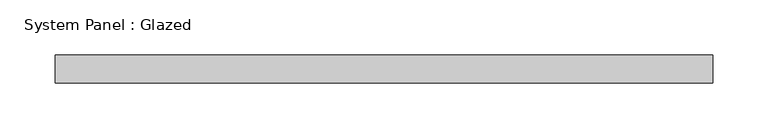
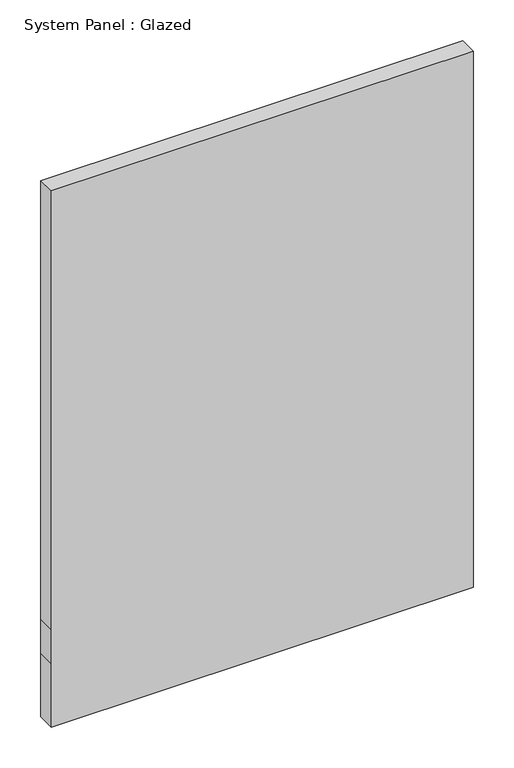
"""IFC4 building model written with IfcOpenShell, lengths in millimetres: plate geometry, System Panel : Glazed."""

from ifc_helpers import new_model, si_unit, frame, origin, place, context, project, spatial, polyline, outline, extrude, source, transform, mapped, element, save


def system_panel_glazed_ba2d6641(model_context):
    return source(origin(), model_context, "Body", "SweptSolid", [
        extrude(outline(polyline([(0.0, -298.45), (0.0, 298.45), (95.25, 298.45), (146.05, 298.45), (802.1539078, 298.45), (802.1539078, -298.45), (146.05, -298.45), (95.25, -298.45), (0.0, -298.45)])), frame((0.0, 19.05, 0.0), z_axis=(0.0, 1.0, 0.0), x_axis=(0.0, 0.0, 1.0)), (0.0, 0.0, 1.0), 25.4),
    ])


if __name__ == "__main__":
    model = new_model("IFC4")
    model_context = context("Model", 3, world=origin())
    ifc_project = project(units=[si_unit("LENGTHUNIT", "METRE", prefix="MILLI")], contexts=[model_context])
    site = spatial("IfcSite", under=ifc_project)
    building = spatial("IfcBuilding", under=site)
    placement = place(None, origin())
    system_panel_glazed_shape = system_panel_glazed_ba2d6641(model_context)
    element("IfcPlate", 1, ObjectType="System Panel : Glazed", at=placement, inside=building, context=model_context, shape_type="MappedRepresentation", body=[
        mapped(system_panel_glazed_shape, transform((0.0, 0.0, 0.0), x_axis=(1.0, 0.0, 0.0), y_axis=(0.0, 1.0, 0.0), z_axis=(0.0, 0.0, 1.0))),
    ])
    save(model, "model.ifc")

# Revit data of these elements
# Type "System Panel : Glazed"
#   Construction Type Id = "GSP4R"
#   Analytic Construction = "1/8 in Pilkington single glazing"
#   Visual Light Transmittance = 0.9
#   Solar Heat Gain Coefficient = 0.86
#   Heat Transfer Coefficient (U) = 1.18115 BTU/(h·ft²·°F)
#   Define Thermal Properties by = 1
# Element 1 (IfcPlate, "System Panel : Glazed")
#   Materials on its faces: "Glass"
# Materials
#   "Glass": class "Glass", colour RGB 0 128 192, transparency 0.75, Description = "Soda Lime Glass", Cost = 0
